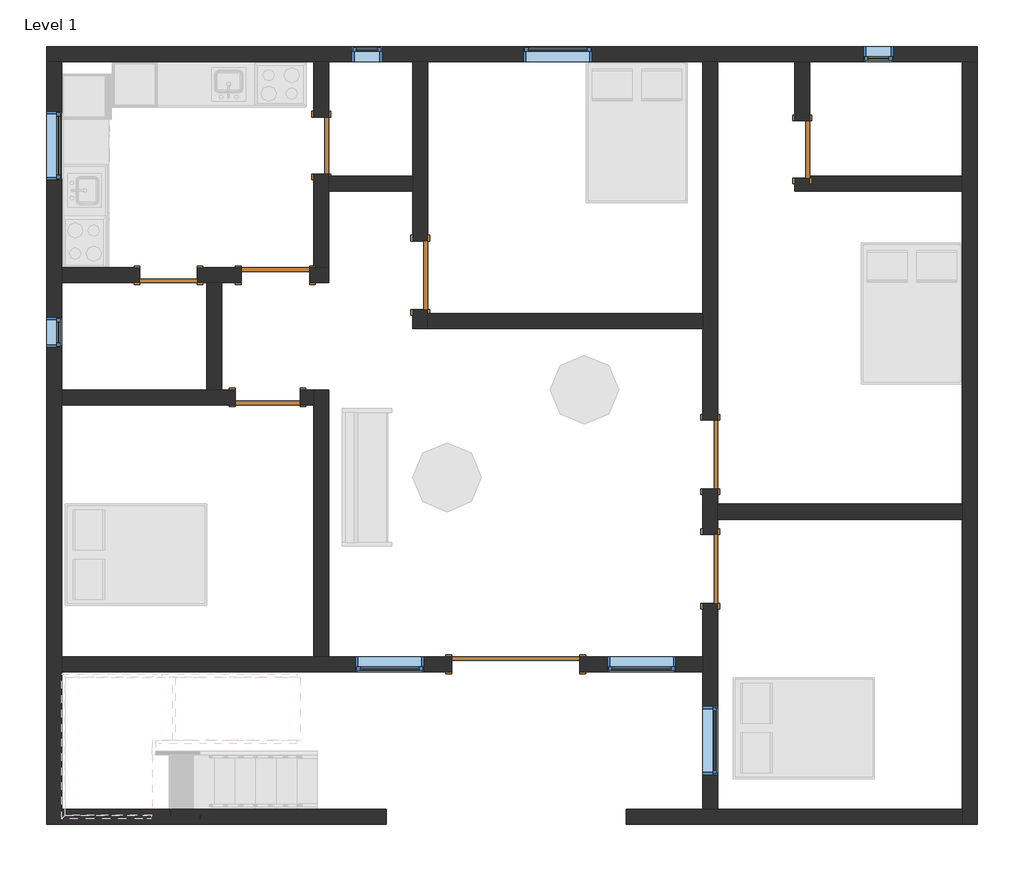
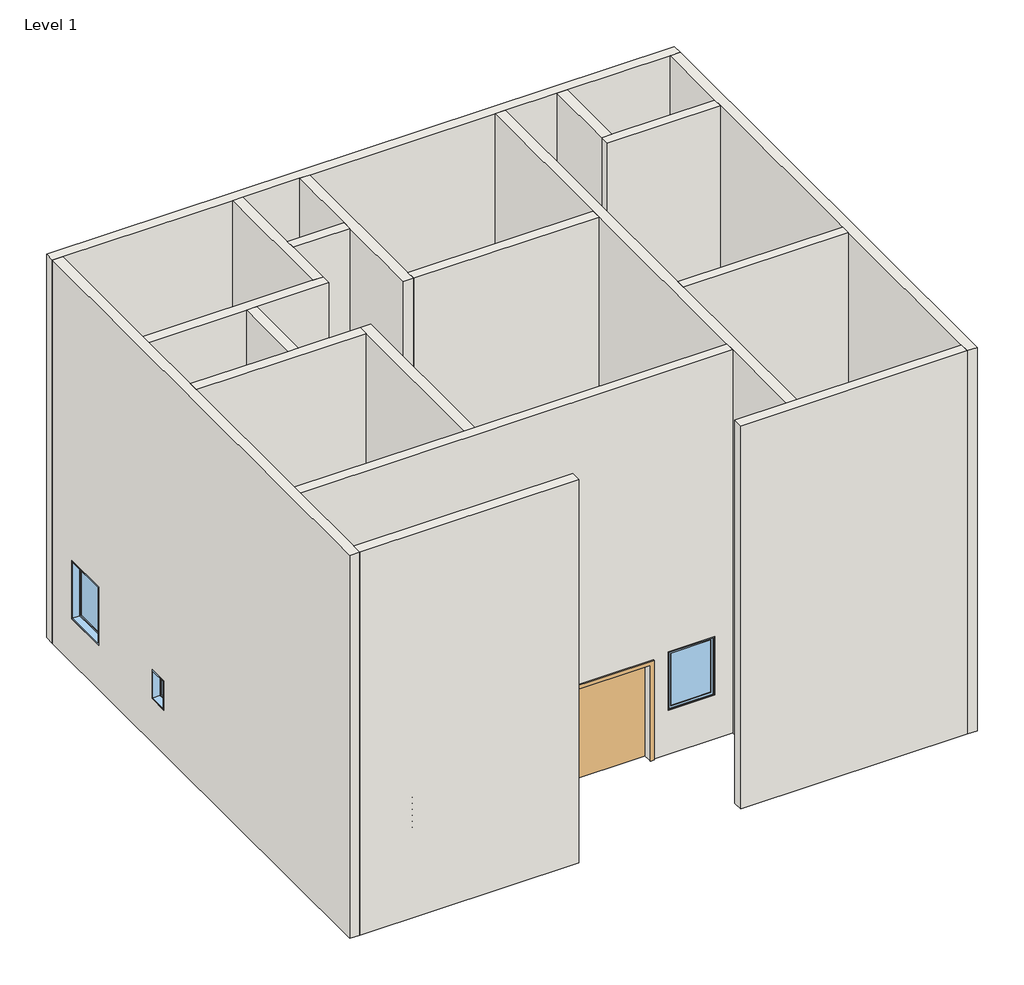
# One storey, part 1 of 4: 18 walls, 9 doors, 8 windows.
"""IFC4 building model written with IfcOpenShell, lengths in millimetres."""

from ifc_helpers import new_model, si_unit, frame, origin, origin_with_axes, place, context, project, spatial, polyline, outline, extrude, faceted_brep, transform, mapped, element, save
from components import m_door_double_flush_panel_double_acting_1700_x_2000mm_0a6d9c7f, m_single_flush_0762_x_2032mm_0c256fab, m_single_flush_0762_x_2032mm_7341a4fb, m_single_flush_0864_x_2032mm_0516f16c, m_single_flush_0915_x_2032mm_7267827e, m_single_flush_0915_x_2134mm_6a9e8738, m_single_flush_0915_x_2134mm_727434cd, m_fixed_0406_x_0610mm_8205b201, m_fixed_0915_x_0610mm_70a843a6, m_fixed_0915_x_1220mm_488fb2fb

model = new_model("IFC4")

# Units and contexts
model_context = context("Model", 3, world=origin())
ifc_project = project(units=[si_unit("LENGTHUNIT", "METRE", prefix="MILLI")], contexts=[model_context])

# Site, building, storey
site = spatial("IfcSite", under=ifc_project)
building = spatial("IfcBuilding", under=site)
storey = spatial("IfcBuildingStorey", under=building, Name="Level 1", Elevation=0.0)

# Doors
placement = place(None, origin())
m_door_double_flush_panel_double_acting_1700_x_2000mm_shape = m_door_double_flush_panel_double_acting_1700_x_2000mm_0a6d9c7f(model_context)
element("IfcDoor", 1, ObjectType="M_Door-Double-Flush_Panel-Double-Acting : 1700 x 2000mm", at=placement, inside=storey, context=model_context, shape_type="MappedRepresentation", body=[
    mapped(m_door_double_flush_panel_double_acting_1700_x_2000mm_shape, transform((-4513.6870075, 3420.4865734, 0.0), x_axis=(1.0, 0.0, 0.0), y_axis=(0.0, 1.0, 0.0), z_axis=(0.0, 0.0, 1.0))),
])
m_single_flush_0762_x_2032mm_shape = m_single_flush_0762_x_2032mm_0c256fab(model_context)
element("IfcDoor", 2, ObjectType="M_Single-Flush : 0762 x 2032mm", at=placement, inside=storey, context=model_context, shape_type="MappedRepresentation", body=[
    mapped(m_single_flush_0762_x_2032mm_shape, transform((-7102.8870075, 10329.2865734, 0.0), x_axis=(0.0, -1.0, 0.0), y_axis=(1.0, 0.0, 0.0), z_axis=(0.0, 0.0, 1.0))),
])
element("IfcDoor", 3, ObjectType="M_Single-Flush : 0762 x 2032mm", at=placement, inside=storey, context=model_context, shape_type="MappedRepresentation", body=[
    mapped(m_single_flush_0762_x_2032mm_shape, transform((-700.4870075, 10278.4865734, 0.0), x_axis=(0.0, -1.0, 0.0), y_axis=(1.0, 0.0, 0.0), z_axis=(0.0, 0.0, 1.0))),
])
m_single_flush_0762_x_2032mm_2_shape = m_single_flush_0762_x_2032mm_7341a4fb(model_context)
element("IfcDoor", 4, ObjectType="M_Single-Flush : 0762 x 2032mm", at=placement, inside=storey, context=model_context, shape_type="MappedRepresentation", body=[
    mapped(m_single_flush_0762_x_2032mm_2_shape, transform((-9136.4870075, 8602.0865734, 0.0), x_axis=(1.0, 0.0, 0.0), y_axis=(0.0, 1.0, 0.0), z_axis=(0.0, 0.0, 1.0))),
])
m_single_flush_0864_x_2032mm_shape = m_single_flush_0864_x_2032mm_0516f16c(model_context)
element("IfcDoor", 5, ObjectType="M_Single-Flush : 0864 x 2032mm", at=placement, inside=storey, context=model_context, shape_type="MappedRepresentation", body=[
    mapped(m_single_flush_0864_x_2032mm_shape, transform((-7815.6870075, 6976.4865734, 0.0), x_axis=(1.0, 0.0, 0.0), y_axis=(0.0, 1.0, 0.0), z_axis=(0.0, 0.0, 1.0))),
])
m_single_flush_0915_x_2032mm_shape = m_single_flush_0915_x_2032mm_7267827e(model_context)
element("IfcDoor", 6, ObjectType="M_Single-Flush : 0915 x 2032mm", at=placement, inside=storey, context=model_context, shape_type="MappedRepresentation", body=[
    mapped(m_single_flush_0915_x_2032mm_shape, transform((-5783.6870075, 8602.0865734, 0.0), x_axis=(0.0, -1.0, 0.0), y_axis=(1.0, 0.0, 0.0), z_axis=(0.0, 0.0, 1.0))),
])
m_single_flush_0915_x_2134mm_shape = m_single_flush_0915_x_2134mm_6a9e8738(model_context)
element("IfcDoor", 7, ObjectType="M_Single-Flush : 0915 x 2134mm", at=placement, inside=storey, context=model_context, shape_type="MappedRepresentation", body=[
    mapped(m_single_flush_0915_x_2134mm_shape, transform((-7712.4870075, 8602.0865734, 0.0), x_axis=(1.0, 0.0, 0.0), y_axis=(0.0, 1.0, 0.0), z_axis=(0.0, 0.0, 1.0))),
])
element("IfcDoor", 8, ObjectType="M_Single-Flush : 0915 x 2134mm", at=placement, inside=storey, context=model_context, shape_type="MappedRepresentation", body=[
    mapped(m_single_flush_0915_x_2134mm_shape, transform((-1922.8870075, 6214.4865734, 0.0), x_axis=(0.0, -1.0, 0.0), y_axis=(1.0, 0.0, 0.0), z_axis=(0.0, 0.0, 1.0))),
])
m_single_flush_0915_x_2134mm_2_shape = m_single_flush_0915_x_2134mm_727434cd(model_context)
element("IfcDoor", 9, ObjectType="M_Single-Flush : 0915 x 2134mm", at=placement, inside=storey, context=model_context, shape_type="MappedRepresentation", body=[
    mapped(m_single_flush_0915_x_2134mm_2_shape, transform((-1922.8870075, 4690.4865734, 0.0), x_axis=(0.0, 1.0, 0.0), y_axis=(-1.0, 0.0, 0.0), z_axis=(0.0, 0.0, 1.0))),
])

# Walls
element("IfcWall", 10, ObjectType="Generic - 200mm", at=placement, inside=storey, context=model_context, shape_type="Brep", body=[
    faceted_brep([(-10758.8870075, 11448.4865734, 0.0), (-10558.8870075, 11448.4865734, 0.0), (-7202.8870075, 11448.4865734, 0.0), (-7002.8870075, 11448.4865734, 0.0), (-5883.6870075, 11448.4865734, 0.0), (-5683.6870075, 11448.4865734, 0.0), (-2022.8870075, 11448.4865734, 0.0), (-1822.8870075, 11448.4865734, 0.0), (-800.4870075, 11448.4865734, 0.0), (-600.4870075, 11448.4865734, 0.0), (1433.1129925, 11448.4865734, 0.0), (1633.1129925, 11448.4865734, 0.0), (1633.1129925, 11448.4865734, 8000.0), (1433.1129925, 11448.4865734, 8000.0), (-600.4870075, 11448.4865734, 8000.0), (-800.4870075, 11448.4865734, 8000.0), (-1822.8870075, 11448.4865734, 8000.0), (-2022.8870075, 11448.4865734, 8000.0), (-5683.6870075, 11448.4865734, 8000.0), (-5883.6870075, 11448.4865734, 8000.0), (-7002.8870075, 11448.4865734, 8000.0), (-7202.8870075, 11448.4865734, 8000.0), (-10558.8870075, 11448.4865734, 8000.0), (-10758.8870075, 11448.4865734, 8000.0), (-4412.3870075, 11448.4865734, 915.0), (-4412.3870075, 11448.4865734, 1525.0), (-3497.3870075, 11448.4865734, 1525.0), (-3497.3870075, 11448.4865734, 915.0), (-6696.2870075, 11448.4865734, 915.0), (-6696.2870075, 11448.4865734, 1525.0), (-6290.2870075, 11448.4865734, 1525.0), (-6290.2870075, 11448.4865734, 915.0), (516.9129925, 11448.4865734, 915.0), (110.9129925, 11448.4865734, 915.0), (110.9129925, 11448.4865734, 1525.0), (516.9129925, 11448.4865734, 1525.0), (-10758.8870075, 11648.4865734, 0.0), (-10758.8870075, 11648.4865734, 8000.0), (1633.1129925, 11648.4865734, 8000.0), (1633.1129925, 11648.4865734, 0.0), (-4412.3870075, 11648.4865734, 915.0), (-3497.3870075, 11648.4865734, 915.0), (-3497.3870075, 11648.4865734, 1525.0), (-4412.3870075, 11648.4865734, 1525.0), (-6696.2870075, 11648.4865734, 915.0), (-6290.2870075, 11648.4865734, 915.0), (-6290.2870075, 11648.4865734, 1525.0), (-6696.2870075, 11648.4865734, 1525.0), (516.9129925, 11648.4865734, 915.0), (516.9129925, 11648.4865734, 1525.0), (110.9129925, 11648.4865734, 1525.0), (110.9129925, 11648.4865734, 915.0)], [[[0, 1, 2, 3, 4, 5, 6, 7, 8, 9, 10, 11, 12, 13, 14, 15, 16, 17, 18, 19, 20, 21, 22, 23], [24, 25, 26, 27], [28, 29, 30, 31], [32, 33, 34, 35]], [[36, 37, 38, 39], [40, 41, 42, 43], [44, 45, 46, 47], [48, 49, 50, 51]], [[11, 10, 9, 8, 7, 6, 5, 4, 3, 2, 1, 0, 36, 39]], [[23, 22, 21, 20, 19, 18, 17, 16, 15, 14, 13, 12, 38, 37]], [[12, 11, 39, 38]], [[0, 23, 37, 36]], [[25, 24, 40, 43]], [[26, 25, 43, 42]], [[27, 26, 42, 41]], [[24, 27, 41, 40]], [[29, 28, 44, 47]], [[30, 29, 47, 46]], [[31, 30, 46, 45]], [[28, 31, 45, 44]], [[49, 48, 32, 35]], [[50, 49, 35, 34]], [[51, 50, 34, 33]], [[48, 51, 33, 32]]]),
])
element("IfcWall", 11, ObjectType="Generic - 200mm", at=placement, inside=storey, context=model_context, shape_type="Brep", body=[
    faceted_brep([(1433.1129925, 11448.4865734, 0.0), (1433.1129925, 9921.2865734, 0.0), (1433.1129925, 9721.2865734, 0.0), (1433.1129925, 5552.4865734, 0.0), (1433.1129925, 5352.4865734, 0.0), (1433.1129925, 1488.4865734, 0.0), (1433.1129925, 1288.4865734, 0.0), (1433.1129925, 1288.4865734, 8000.0), (1433.1129925, 1488.4865734, 8000.0), (1433.1129925, 5352.4865734, 8000.0), (1433.1129925, 5552.4865734, 8000.0), (1433.1129925, 9721.2865734, 8000.0), (1433.1129925, 9921.2865734, 8000.0), (1433.1129925, 11448.4865734, 8000.0), (1633.1129925, 11448.4865734, 0.0), (1633.1129925, 11448.4865734, 8000.0), (1633.1129925, 1288.4865734, 8000.0), (1633.1129925, 1288.4865734, 0.0)], [[[0, 1, 2, 3, 4, 5, 6, 7, 8, 9, 10, 11, 12, 13]], [[14, 15, 16, 17]], [[6, 5, 4, 3, 2, 1, 0, 14, 17]], [[13, 12, 11, 10, 9, 8, 7, 16, 15]], [[0, 13, 15, 14]], [[7, 6, 17, 16]]]),
])
element("IfcWall", 12, ObjectType="Generic - 200mm", at=placement, inside=storey, context=model_context, shape_type="Brep", body=[
    faceted_brep([(-10558.8870075, 1288.4865734, 0.0), (-10558.8870075, 1488.4865734, 0.0), (-10558.8870075, 3320.4865734, 0.0), (-10558.8870075, 3520.4865734, 0.0), (-10558.8870075, 6876.4865734, 0.0), (-10558.8870075, 7076.4865734, 0.0), (-10558.8870075, 8502.0865734, 0.0), (-10558.8870075, 8702.0865734, 0.0), (-10558.8870075, 11448.4865734, 0.0), (-10558.8870075, 11448.4865734, 8000.0), (-10558.8870075, 8702.0865734, 8000.0), (-10558.8870075, 8502.0865734, 8000.0), (-10558.8870075, 7076.4865734, 8000.0), (-10558.8870075, 6876.4865734, 8000.0), (-10558.8870075, 3520.4865734, 8000.0), (-10558.8870075, 3320.4865734, 8000.0), (-10558.8870075, 1488.4865734, 8000.0), (-10558.8870075, 1288.4865734, 8000.0), (-10558.8870075, 10786.7865734, 915.0), (-10558.8870075, 9871.7865734, 915.0), (-10558.8870075, 9871.7865734, 2135.0), (-10558.8870075, 10786.7865734, 2135.0), (-10558.8870075, 8043.0865734, 915.0), (-10558.8870075, 7637.0865734, 915.0), (-10558.8870075, 7637.0865734, 1525.0), (-10558.8870075, 8043.0865734, 1525.0), (-10758.8870075, 1288.4865734, 0.0), (-10758.8870075, 1288.4865734, 8000.0), (-10758.8870075, 11448.4865734, 8000.0), (-10758.8870075, 11448.4865734, 0.0), (-10758.8870075, 10786.7865734, 915.0), (-10758.8870075, 10786.7865734, 2135.0), (-10758.8870075, 9871.7865734, 2135.0), (-10758.8870075, 9871.7865734, 915.0), (-10758.8870075, 8043.0865734, 915.0), (-10758.8870075, 8043.0865734, 1525.0), (-10758.8870075, 7637.0865734, 1525.0), (-10758.8870075, 7637.0865734, 915.0)], [[[0, 1, 2, 3, 4, 5, 6, 7, 8, 9, 10, 11, 12, 13, 14, 15, 16, 17], [18, 19, 20, 21], [22, 23, 24, 25]], [[26, 27, 28, 29], [30, 31, 32, 33], [34, 35, 36, 37]], [[8, 7, 6, 5, 4, 3, 2, 1, 0, 26, 29]], [[17, 16, 15, 14, 13, 12, 11, 10, 9, 28, 27]], [[9, 8, 29, 28]], [[31, 30, 18, 21]], [[32, 31, 21, 20]], [[33, 32, 20, 19]], [[30, 33, 19, 18]], [[35, 34, 22, 25]], [[36, 35, 25, 24]], [[37, 36, 24, 23]], [[34, 37, 23, 22]], [[0, 17, 27, 26]]]),
])
element("IfcWall", 13, ObjectType="Generic - 200mm", at=placement, inside=storey, context=model_context, shape_type="Brep", body=[
    faceted_brep([(-8755.4870075, 8502.0865734, 2032.0), (-8755.4870075, 8502.0865734, 0.0), (-8626.8870075, 8502.0865734, 0.0), (-8426.8870075, 8502.0865734, 0.0), (-8169.9870075, 8502.0865734, 0.0), (-8169.9870075, 8502.0865734, 2134.0), (-7254.9870075, 8502.0865734, 2134.0), (-7254.9870075, 8502.0865734, 0.0), (-7002.8870075, 8502.0865734, 0.0), (-7002.8870075, 8502.0865734, 8000.0), (-8426.8870075, 8502.0865734, 8000.0), (-8626.8870075, 8502.0865734, 8000.0), (-10558.8870075, 8502.0865734, 8000.0), (-10558.8870075, 8502.0865734, 0.0), (-9517.4870075, 8502.0865734, 0.0), (-9517.4870075, 8502.0865734, 2032.0), (-8169.9870075, 8702.0865734, 0.0), (-8755.4870075, 8702.0865734, 0.0), (-8755.4870075, 8702.0865734, 2032.0), (-9517.4870075, 8702.0865734, 2032.0), (-9517.4870075, 8702.0865734, 0.0), (-10558.8870075, 8702.0865734, 0.0), (-10558.8870075, 8702.0865734, 8000.0), (-7202.8870075, 8702.0865734, 8000.0), (-7002.8870075, 8702.0865734, 8000.0), (-7002.8870075, 8702.0865734, 0.0), (-7202.8870075, 8702.0865734, 0.0), (-7254.9870075, 8702.0865734, 0.0), (-7254.9870075, 8702.0865734, 2134.0), (-8169.9870075, 8702.0865734, 2134.0)], [[[0, 1, 2, 3, 4, 5, 6, 7, 8, 9, 10, 11, 12, 13, 14, 15]], [[16, 17, 18, 19, 20, 21, 22, 23, 24, 25, 26, 27, 28, 29]], [[8, 7, 27, 26, 25]], [[14, 13, 21, 20]], [[4, 3, 2, 1, 17, 16]], [[12, 11, 10, 9, 24, 23, 22]], [[13, 12, 22, 21]], [[9, 8, 25, 24]], [[28, 27, 7, 6]], [[29, 28, 6, 5]], [[16, 29, 5, 4]], [[18, 17, 1, 0]], [[19, 18, 0, 15]], [[20, 19, 15, 14]]]),
])
element("IfcWall", 14, ObjectType="Generic - 200mm", at=placement, inside=storey, context=model_context, shape_type="Brep", body=[
    faceted_brep([(-7002.8870075, 8702.0865734, 0.0), (-7002.8870075, 9721.2865734, 0.0), (-7002.8870075, 9921.2865734, 0.0), (-7002.8870075, 9948.2865734, 0.0), (-7002.8870075, 9948.2865734, 2032.0), (-7002.8870075, 10710.2865734, 2032.0), (-7002.8870075, 10710.2865734, 0.0), (-7002.8870075, 11448.4865734, 0.0), (-7002.8870075, 11448.4865734, 8000.0), (-7002.8870075, 9921.2865734, 8000.0), (-7002.8870075, 9721.2865734, 8000.0), (-7002.8870075, 8702.0865734, 8000.0), (-7202.8870075, 9948.2865734, 2032.0), (-7202.8870075, 9948.2865734, 0.0), (-7202.8870075, 8702.0865734, 0.0), (-7202.8870075, 8702.0865734, 8000.0), (-7202.8870075, 11448.4865734, 8000.0), (-7202.8870075, 11448.4865734, 0.0), (-7202.8870075, 10710.2865734, 0.0), (-7202.8870075, 10710.2865734, 2032.0)], [[[0, 1, 2, 3, 4, 5, 6, 7, 8, 9, 10, 11]], [[12, 13, 14, 15, 16, 17, 18, 19]], [[18, 17, 7, 6]], [[14, 13, 3, 2, 1, 0]], [[11, 10, 9, 8, 16, 15]], [[0, 11, 15, 14]], [[8, 7, 17, 16]], [[4, 3, 13, 12]], [[5, 4, 12, 19]], [[6, 5, 19, 18]]]),
])
element("IfcWall", 15, ObjectType="Generic - 200mm", at=placement, inside=storey, context=model_context, shape_type="SweptSolid", body=[
    extrude(outline(polyline([(-5883.6870075, 9721.2865734), (-7002.8870075, 9721.2865734), (-7002.8870075, 9921.2865734), (-5883.6870075, 9921.2865734), (-5883.6870075, 9721.2865734)])), origin_with_axes(), (0.0, 0.0, 1.0), 8000.0),
])
element("IfcWall", 16, ObjectType="Generic - 200mm", at=placement, inside=storey, context=model_context, shape_type="Brep", body=[
    faceted_brep([(-5683.6870075, 7892.4865734, 0.0), (-5683.6870075, 8092.4865734, 0.0), (-5683.6870075, 8144.5865734, 0.0), (-5683.6870075, 8144.5865734, 2032.0), (-5683.6870075, 9059.5865734, 2032.0), (-5683.6870075, 9059.5865734, 0.0), (-5683.6870075, 11448.4865734, 0.0), (-5683.6870075, 11448.4865734, 8000.0), (-5683.6870075, 8092.4865734, 8000.0), (-5683.6870075, 7892.4865734, 8000.0), (-5883.6870075, 8144.5865734, 2032.0), (-5883.6870075, 8144.5865734, 0.0), (-5883.6870075, 7892.4865734, 0.0), (-5883.6870075, 7892.4865734, 8000.0), (-5883.6870075, 9721.2865734, 8000.0), (-5883.6870075, 9921.2865734, 8000.0), (-5883.6870075, 11448.4865734, 8000.0), (-5883.6870075, 11448.4865734, 0.0), (-5883.6870075, 9921.2865734, 0.0), (-5883.6870075, 9721.2865734, 0.0), (-5883.6870075, 9059.5865734, 0.0), (-5883.6870075, 9059.5865734, 2032.0)], [[[0, 1, 2, 3, 4, 5, 6, 7, 8, 9]], [[10, 11, 12, 13, 14, 15, 16, 17, 18, 19, 20, 21]], [[12, 11, 2, 1, 0]], [[20, 19, 18, 17, 6, 5]], [[9, 8, 7, 16, 15, 14, 13]], [[7, 6, 17, 16]], [[0, 9, 13, 12]], [[3, 2, 11, 10]], [[4, 3, 10, 21]], [[5, 4, 21, 20]]]),
])
element("IfcWall", 17, ObjectType="Generic - 200mm", at=placement, inside=storey, context=model_context, shape_type="SweptSolid", body=[
    extrude(outline(polyline([(-2022.8870075, 7892.4865734), (-5683.6870075, 7892.4865734), (-5683.6870075, 8092.4865734), (-2022.8870075, 8092.4865734), (-2022.8870075, 7892.4865734)])), origin_with_axes(), (0.0, 0.0, 1.0), 8000.0),
])
element("IfcWall", 18, ObjectType="Generic - 200mm", at=placement, inside=storey, context=model_context, shape_type="Brep", body=[
    faceted_brep([(-800.4870075, 9921.2865734, 8000.0), (-600.4870075, 9921.2865734, 8000.0), (1433.1129925, 9921.2865734, 8000.0), (1433.1129925, 9921.2865734, 0.0), (-600.4870075, 9921.2865734, 0.0), (-600.4870075, 9921.2865734, 2032.0), (-800.4870075, 9921.2865734, 2032.0), (-800.4870075, 9721.2865734, 0.0), (1433.1129925, 9721.2865734, 0.0), (1433.1129925, 9721.2865734, 8000.0), (-800.4870075, 9721.2865734, 8000.0), (-800.4870075, 9897.4865734, 0.0), (-600.4870075, 9897.4865734, 0.0), (-800.4870075, 9897.4865734, 2032.0), (-600.4870075, 9897.4865734, 2032.0)], [[[0, 1, 2, 3, 4, 5, 6]], [[7, 8, 9, 10]], [[8, 7, 11, 12, 4, 3]], [[2, 1, 0, 10, 9]], [[3, 2, 9, 8]], [[7, 10, 0, 6, 13, 11]], [[12, 14, 5, 4]], [[14, 12, 11, 13]], [[14, 13, 6, 5]]]),
])
element("IfcWall", 19, ObjectType="Generic - 200mm", at=placement, inside=storey, context=model_context, shape_type="SweptSolid", body=[
    extrude(outline(polyline([(9921.2865734, 8000.0), (11448.4865734, 8000.0), (11448.4865734, 0.0), (10659.4865734, 0.0), (10659.4865734, 2032.0), (9921.2865734, 2032.0), (9921.2865734, 8000.0)])), frame((-800.4870075, 0.0, 0.0), z_axis=(1.0, 0.0, 0.0), x_axis=(0.0, 1.0, 0.0)), (0.0, 0.0, 1.0), 200.0),
])
element("IfcWall", 20, ObjectType="Generic - 200mm", at=placement, inside=storey, context=model_context, shape_type="Brep", body=[
    faceted_brep([(-1822.8870075, 5147.9865734, 2134.0), (-1822.8870075, 5147.9865734, 0.0), (-1822.8870075, 5352.4865734, 0.0), (-1822.8870075, 5552.4865734, 0.0), (-1822.8870075, 5756.9865734, 0.0), (-1822.8870075, 5756.9865734, 2134.0), (-1822.8870075, 6671.9865734, 2134.0), (-1822.8870075, 6671.9865734, 0.0), (-1822.8870075, 11448.4865734, 0.0), (-1822.8870075, 11448.4865734, 8000.0), (-1822.8870075, 5552.4865734, 8000.0), (-1822.8870075, 5352.4865734, 8000.0), (-1822.8870075, 1488.4865734, 8000.0), (-1822.8870075, 1488.4865734, 0.0), (-1822.8870075, 4232.9865734, 0.0), (-1822.8870075, 4232.9865734, 2134.0), (-1822.8870075, 2861.9865734, 915.0), (-1822.8870075, 1946.9865734, 915.0), (-1822.8870075, 1946.9865734, 2135.0), (-1822.8870075, 2861.9865734, 2135.0), (-2022.8870075, 5756.9865734, 0.0), (-2022.8870075, 5147.9865734, 0.0), (-2022.8870075, 5147.9865734, 2134.0), (-2022.8870075, 4232.9865734, 2134.0), (-2022.8870075, 4232.9865734, 0.0), (-2022.8870075, 3520.4865734, 0.0), (-2022.8870075, 3320.4865734, 0.0), (-2022.8870075, 1488.4865734, 0.0), (-2022.8870075, 1488.4865734, 8000.0), (-2022.8870075, 3320.4865734, 8000.0), (-2022.8870075, 3520.4865734, 8000.0), (-2022.8870075, 7892.4865734, 8000.0), (-2022.8870075, 8092.4865734, 8000.0), (-2022.8870075, 11448.4865734, 8000.0), (-2022.8870075, 11448.4865734, 0.0), (-2022.8870075, 8092.4865734, 0.0), (-2022.8870075, 7892.4865734, 0.0), (-2022.8870075, 6671.9865734, 0.0), (-2022.8870075, 6671.9865734, 2134.0), (-2022.8870075, 5756.9865734, 2134.0), (-2022.8870075, 2861.9865734, 915.0), (-2022.8870075, 2861.9865734, 2135.0), (-2022.8870075, 1946.9865734, 2135.0), (-2022.8870075, 1946.9865734, 915.0)], [[[0, 1, 2, 3, 4, 5, 6, 7, 8, 9, 10, 11, 12, 13, 14, 15], [16, 17, 18, 19]], [[20, 21, 22, 23, 24, 25, 26, 27, 28, 29, 30, 31, 32, 33, 34, 35, 36, 37, 38, 39], [40, 41, 42, 43]], [[37, 36, 35, 34, 8, 7]], [[14, 13, 27, 26, 25, 24]], [[4, 3, 2, 1, 21, 20]], [[12, 11, 10, 9, 33, 32, 31, 30, 29, 28]], [[9, 8, 34, 33]], [[5, 4, 20, 39]], [[6, 5, 39, 38]], [[7, 6, 38, 37]], [[22, 21, 1, 0]], [[23, 22, 0, 15]], [[24, 23, 15, 14]], [[41, 40, 16, 19]], [[42, 41, 19, 18]], [[43, 42, 18, 17]], [[40, 43, 17, 16]], [[13, 12, 28, 27]]]),
])
element("IfcWall", 21, ObjectType="Generic - 200mm", at=placement, inside=storey, context=model_context, shape_type="SweptSolid", body=[
    extrude(outline(polyline([(1433.1129925, 5352.4865734), (-1822.8870075, 5352.4865734), (-1822.8870075, 5552.4865734), (1433.1129925, 5552.4865734), (1433.1129925, 5352.4865734)])), origin_with_axes(), (0.0, 0.0, 1.0), 8000.0),
])
element("IfcWall", 22, ObjectType="Generic - 200mm", at=placement, inside=storey, context=model_context, shape_type="Brep", body=[
    faceted_brep([(-7383.6870075, 6876.4865734, 2032.0), (-7383.6870075, 6876.4865734, 0.0), (-7204.4870075, 6876.4865734, 0.0), (-7204.4870075, 6876.4865734, 8000.0), (-10558.8870075, 6876.4865734, 8000.0), (-10558.8870075, 6876.4865734, 0.0), (-8247.6870075, 6876.4865734, 0.0), (-8247.6870075, 6876.4865734, 2032.0), (-7204.4870075, 7076.4865734, 0.0), (-7383.6870075, 7076.4865734, 0.0), (-7383.6870075, 7076.4865734, 2032.0), (-8247.6870075, 7076.4865734, 2032.0), (-8247.6870075, 7076.4865734, 0.0), (-8426.8870075, 7076.4865734, 0.0), (-8626.8870075, 7076.4865734, 0.0), (-10558.8870075, 7076.4865734, 0.0), (-10558.8870075, 7076.4865734, 8000.0), (-8626.8870075, 7076.4865734, 8000.0), (-8426.8870075, 7076.4865734, 8000.0), (-7204.4870075, 7076.4865734, 8000.0)], [[[0, 1, 2, 3, 4, 5, 6, 7]], [[8, 9, 10, 11, 12, 13, 14, 15, 16, 17, 18, 19]], [[6, 5, 15, 14, 13, 12]], [[2, 1, 9, 8]], [[4, 3, 19, 18, 17, 16]], [[5, 4, 16, 15]], [[3, 2, 8, 19]], [[10, 9, 1, 0]], [[11, 10, 0, 7]], [[12, 11, 7, 6]]]),
])
element("IfcWall", 23, ObjectType="Generic - 200mm", at=placement, inside=storey, context=model_context, shape_type="SweptSolid", body=[
    extrude(outline(polyline([(-8426.8870075, 8502.0865734), (-8426.8870075, 7076.4865734), (-8626.8870075, 7076.4865734), (-8626.8870075, 8502.0865734), (-8426.8870075, 8502.0865734)])), origin_with_axes(), (0.0, 0.0, 1.0), 8000.0),
])
element("IfcWall", 24, ObjectType="Generic - 200mm", at=placement, inside=storey, context=model_context, shape_type="Brep", body=[
    faceted_brep([(-2022.8870075, 3320.4865734, 8000.0), (-10558.8870075, 3320.4865734, 8000.0), (-10558.8870075, 3320.4865734, 0.0), (-5363.6870075, 3320.4865734, 0.0), (-5363.6870075, 3320.4865734, 2000.0), (-3663.6870075, 3320.4865734, 2000.0), (-3663.6870075, 3320.4865734, 0.0), (-2022.8870075, 3320.4865734, 0.0), (-5732.5870075, 3320.4865734, 915.0), (-6647.5870075, 3320.4865734, 915.0), (-6647.5870075, 3320.4865734, 2135.0), (-5732.5870075, 3320.4865734, 2135.0), (-2379.7870075, 3320.4865734, 915.0), (-3294.7870075, 3320.4865734, 915.0), (-3294.7870075, 3320.4865734, 2135.0), (-2379.7870075, 3320.4865734, 2135.0), (-10558.8870075, 3520.4865734, 8000.0), (-7204.4870075, 3520.4865734, 8000.0), (-7004.4870075, 3520.4865734, 8000.0), (-2022.8870075, 3520.4865734, 8000.0), (-2022.8870075, 3520.4865734, 0.0), (-3663.6870075, 3520.4865734, 0.0), (-3663.6870075, 3520.4865734, 2000.0), (-5363.6870075, 3520.4865734, 2000.0), (-5363.6870075, 3520.4865734, 0.0), (-7004.4870075, 3520.4865734, 0.0), (-7204.4870075, 3520.4865734, 0.0), (-10558.8870075, 3520.4865734, 0.0), (-5732.5870075, 3520.4865734, 915.0), (-5732.5870075, 3520.4865734, 2135.0), (-6647.5870075, 3520.4865734, 2135.0), (-6647.5870075, 3520.4865734, 915.0), (-2379.7870075, 3520.4865734, 915.0), (-2379.7870075, 3520.4865734, 2135.0), (-3294.7870075, 3520.4865734, 2135.0), (-3294.7870075, 3520.4865734, 915.0)], [[[0, 1, 2, 3, 4, 5, 6, 7], [8, 9, 10, 11], [12, 13, 14, 15]], [[16, 17, 18, 19, 20, 21, 22, 23, 24, 25, 26, 27], [28, 29, 30, 31], [32, 33, 34, 35]], [[2, 27, 26, 25, 24, 3]], [[20, 7, 6, 21]], [[1, 0, 19, 18, 17, 16]], [[2, 1, 16, 27]], [[0, 7, 20, 19]], [[5, 22, 21, 6]], [[22, 5, 4, 23]], [[23, 4, 3, 24]], [[29, 28, 8, 11]], [[30, 29, 11, 10]], [[31, 30, 10, 9]], [[28, 31, 9, 8]], [[33, 32, 12, 15]], [[34, 33, 15, 14]], [[35, 34, 14, 13]], [[32, 35, 13, 12]]]),
])
element("IfcWall", 25, ObjectType="Generic - 200mm", at=placement, inside=storey, context=model_context, shape_type="Brep", body=[
    faceted_brep([(-7004.4870075, 3520.4865734, 0.0), (-7004.4870075, 7076.4865734, 0.0), (-7004.4870075, 7076.4865734, 8000.0), (-7004.4870075, 3520.4865734, 8000.0), (-7204.4870075, 3520.4865734, 0.0), (-7204.4870075, 3520.4865734, 8000.0), (-7204.4870075, 6876.4865734, 8000.0), (-7204.4870075, 7076.4865734, 8000.0), (-7204.4870075, 7076.4865734, 0.0), (-7204.4870075, 6876.4865734, 0.0)], [[[0, 1, 2, 3]], [[4, 5, 6, 7, 8, 9]], [[1, 0, 4, 9, 8]], [[3, 2, 7, 6, 5]], [[0, 3, 5, 4]], [[2, 1, 8, 7]]]),
])
element("IfcWall", 26, ObjectType="Generic - 200mm", at=placement, inside=storey, context=model_context, shape_type="SweptSolid", body=[
    extrude(outline(polyline([(-6239.2870075, 1288.4865734), (-10558.8870075, 1288.4865734), (-10558.8870075, 1488.4865734), (-6239.2870075, 1488.4865734), (-6239.2870075, 1288.4865734)])), origin_with_axes(), (0.0, 0.0, 1.0), 8000.0),
])
element("IfcWall", 27, ObjectType="Generic - 200mm", at=placement, inside=storey, context=model_context, shape_type="Brep", body=[
    faceted_brep([(1433.1129925, 1488.4865734, 0.0), (-1822.8870075, 1488.4865734, 0.0), (-2022.8870075, 1488.4865734, 0.0), (-3038.8870075, 1488.4865734, 0.0), (-3038.8870075, 1488.4865734, 8000.0), (-2022.8870075, 1488.4865734, 8000.0), (-1822.8870075, 1488.4865734, 8000.0), (1433.1129925, 1488.4865734, 8000.0), (1433.1129925, 1288.4865734, 0.0), (1433.1129925, 1288.4865734, 8000.0), (-3038.8870075, 1288.4865734, 8000.0), (-3038.8870075, 1288.4865734, 0.0)], [[[0, 1, 2, 3, 4, 5, 6, 7]], [[8, 9, 10, 11]], [[3, 2, 1, 0, 8, 11]], [[4, 3, 11, 10]], [[7, 6, 5, 4, 10, 9]], [[0, 7, 9, 8]]]),
])

# Windows
m_fixed_0406_x_0610mm_shape = m_fixed_0406_x_0610mm_8205b201(model_context)
element("IfcWindow", 28, ObjectType="M_Fixed : 0406 x 0610mm", at=placement, inside=storey, context=model_context, shape_type="MappedRepresentation", body=[
    mapped(m_fixed_0406_x_0610mm_shape, transform((-6493.2870075, 11535.4865734, 0.0), x_axis=(1.0, 0.0, 0.0), y_axis=(0.0, 1.0, 0.0), z_axis=(0.0, 0.0, 1.0))),
])
element("IfcWindow", 29, ObjectType="M_Fixed : 0406 x 0610mm", at=placement, inside=storey, context=model_context, shape_type="MappedRepresentation", body=[
    mapped(m_fixed_0406_x_0610mm_shape, transform((-10671.8870075, 7840.0865734, 0.0), x_axis=(0.0, -1.0, 0.0), y_axis=(1.0, 0.0, 0.0), z_axis=(0.0, 0.0, 1.0))),
])
element("IfcWindow", 30, ObjectType="M_Fixed : 0406 x 0610mm", at=placement, inside=storey, context=model_context, shape_type="MappedRepresentation", body=[
    mapped(m_fixed_0406_x_0610mm_shape, transform((313.9129925, 11561.4865734, 0.0), x_axis=(-1.0, 0.0, 0.0), y_axis=(0.0, -1.0, 0.0), z_axis=(0.0, 0.0, 1.0))),
])
m_fixed_0915_x_0610mm_shape = m_fixed_0915_x_0610mm_70a843a6(model_context)
element("IfcWindow", 31, ObjectType="M_Fixed : 0915 x 0610mm", at=placement, inside=storey, context=model_context, shape_type="MappedRepresentation", body=[
    mapped(m_fixed_0915_x_0610mm_shape, transform((-3954.8870075, 11535.4865734, 0.0), x_axis=(1.0, 0.0, 0.0), y_axis=(0.0, 1.0, 0.0), z_axis=(0.0, 0.0, 1.0))),
])
m_fixed_0915_x_1220mm_shape = m_fixed_0915_x_1220mm_488fb2fb(model_context)
element("IfcWindow", 32, ObjectType="M_Fixed : 0915 x 1220mm", at=placement, inside=storey, context=model_context, shape_type="MappedRepresentation", body=[
    mapped(m_fixed_0915_x_1220mm_shape, transform((-10671.8870075, 10329.2865734, 0.0), x_axis=(0.0, -1.0, 0.0), y_axis=(1.0, 0.0, 0.0), z_axis=(0.0, 0.0, 1.0))),
])
element("IfcWindow", 33, ObjectType="M_Fixed : 0915 x 1220mm", at=placement, inside=storey, context=model_context, shape_type="MappedRepresentation", body=[
    mapped(m_fixed_0915_x_1220mm_shape, transform((-6190.0870075, 3433.4865734, 0.0), x_axis=(-1.0, 0.0, 0.0), y_axis=(0.0, -1.0, 0.0), z_axis=(0.0, 0.0, 1.0))),
])
element("IfcWindow", 34, ObjectType="M_Fixed : 0915 x 1220mm", at=placement, inside=storey, context=model_context, shape_type="MappedRepresentation", body=[
    mapped(m_fixed_0915_x_1220mm_shape, transform((-2837.2870075, 3433.4865734, 0.0), x_axis=(-1.0, 0.0, 0.0), y_axis=(0.0, -1.0, 0.0), z_axis=(0.0, 0.0, 1.0))),
])
element("IfcWindow", 35, ObjectType="M_Fixed : 0915 x 1220mm", at=placement, inside=storey, context=model_context, shape_type="MappedRepresentation", body=[
    mapped(m_fixed_0915_x_1220mm_shape, transform((-1935.8870075, 2404.4865734, 0.0), x_axis=(0.0, -1.0, 0.0), y_axis=(1.0, 0.0, 0.0), z_axis=(0.0, 0.0, 1.0))),
])

save(model, "model.ifc")

# Revit data of these elements
# Type "M_Door-Double-Flush_Panel-Double-Acting : 1700 x 2000mm"
#   Type Mark = "22"
#   Construction Type Id = "DOOR"
#   Assembly Code = "C1020"
#   Analytic Construction = "Wooden"
#   W = 850 mm
#   Thickness = 50 mm
#   Thermal Resistance (R) = 0.455703 (m²·K)/W
#   Swing Angle [instance default] = 90.00°
#   Heat Transfer Coefficient (U) = 2.19465 W/(m²·K)
#   Height = 2000 mm
#   Trim Projection Ext. = 25 mm
#   Trim Projection Int. = 25 mm
#   Trim Width Ext. = 80 mm
#   Trim Width Int. = 80 mm
#   Width = 1700 mm
#   Define Thermal Properties by = 1
#   Panel Material = Wood - Birch - Solid Stained Light Low Gloss
#   Trim Material = Paint - Sienna
#   Visual Light Transmittance = 0
#   Solar Heat Gain Coefficient = 0
#   Function = (empty or 0)
#   Wall Closure = (empty or 0)
# Type "M_Single-Flush : 0762 x 2032mm"
#   Type Mark = "19"
#   Thickness = 51 mm
#   Height = 2032 mm
#   Trim Projection Ext = 25 mm
#   Trim Projection Int = 25 mm
#   Trim Width = 76 mm
#   Width = 762 mm
#   Door Material = Door - Panel
#   Frame Material = Door - Frame
#   Function = (empty or 0)
#   Wall Closure = (empty or 0)
# Type "M_Single-Flush : 0864 x 2032mm"
#   Type Mark = "21"
#   Thickness = 51 mm
#   Height = 2032 mm
#   Trim Projection Ext = 25 mm
#   Trim Projection Int = 25 mm
#   Trim Width = 76 mm
#   Width = 864 mm
#   Door Material = Door - Panel
#   Frame Material = Door - Frame
#   Function = (empty or 0)
#   Wall Closure = (empty or 0)
# Type "M_Single-Flush : 0915 x 2032mm"
#   Type Mark = "20"
#   Thickness = 51 mm
#   Height = 2032 mm
#   Trim Projection Ext = 25 mm
#   Trim Projection Int = 25 mm
#   Trim Width = 76 mm
#   Width = 915 mm
#   Door Material = Door - Panel
#   Frame Material = Door - Frame
#   Function = (empty or 0)
#   Wall Closure = (empty or 0)
# Type "M_Single-Flush : 0915 x 2134mm"
#   Type Mark = "15"
#   Thickness = 51 mm
#   Height = 2134 mm
#   Trim Projection Ext = 25 mm
#   Trim Projection Int = 25 mm
#   Trim Width = 76 mm
#   Width = 915 mm
#   Door Material = Door - Panel
#   Frame Material = Door - Frame
#   Function = (empty or 0)
#   Wall Closure = (empty or 0)
# Type "Generic - 200mm"
#   Layers, outside or top first: 200 mm no material (function 1)
# Type "M_Fixed : 0406 x 0610mm"
#   Type Mark = "10"
#   Height = 610 mm
#   Default Sill Height = 915 mm
#   Width = 406 mm
#   Window Inset = 19 mm
#   Frame Exterior Material = Sash
#   Frame Interior Material = Sash
#   Glass Pane Material = Glass
#   Sash = Sash
#   Wall Closure = (empty or 0)
# Type "M_Fixed : 0915 x 0610mm"
#   Type Mark = "14"
#   Height = 610 mm
#   Default Sill Height = 915 mm
#   Width = 915 mm
#   Window Inset = 19 mm
#   Frame Exterior Material = Sash
#   Frame Interior Material = Sash
#   Glass Pane Material = Glass
#   Sash = Sash
#   Wall Closure = (empty or 0)
# Type "M_Fixed : 0915 x 1220mm"
#   Type Mark = "15"
#   Height = 1220 mm
#   Default Sill Height = 915 mm
#   Width = 915 mm
#   Window Inset = 19 mm
#   Frame Exterior Material = Sash
#   Frame Interior Material = Sash
#   Glass Pane Material = Glass
#   Sash = Sash
#   Wall Closure = (empty or 0)
# Element 1 (IfcDoor, "M_Door-Double-Flush_Panel-Double-Acting : 1700 x 2000mm")
#   Swing Angle = 90.00°
#   Phase Created = New Construction
#   Materials on its faces: "Paint - Sienna", "Wood - Birch - Solid Stained Light Low Gloss"
# Elements 2, 3, 4 (IfcDoor, "M_Single-Flush : 0762 x 2032mm")
#   Phase Created = New Construction
#   Materials on its faces: "Door - Frame", "Door - Panel"
# Element 5 (IfcDoor, "M_Single-Flush : 0864 x 2032mm")
#   Phase Created = New Construction
#   Materials on its faces: "Door - Frame", "Door - Panel"
# Element 6 (IfcDoor, "M_Single-Flush : 0915 x 2032mm")
#   Phase Created = New Construction
#   Materials on its faces: "Door - Frame", "Door - Panel"
# Elements 7, 8, 9 (IfcDoor, "M_Single-Flush : 0915 x 2134mm")
#   Phase Created = New Construction
#   Materials on its faces: "Door - Frame", "Door - Panel"
# Elements 10, 11, 12, 13, 14, 15, 16, 17, 18, 19, 20, 21, 22, 23, 24, 25, 26, 27 (IfcWall, "Generic - 200mm")
#   Top Offset = 0 mm
#   Base Offset = 0 mm
#   Unconnected Height = 8000 mm
#   wall height = 8000 mm
#   Phase Created = New Construction
#   Base Constraint = Level 1
#   Materials on its faces: "Default Wall"
# Element 28 (IfcWindow, "M_Fixed : 0406 x 0610mm")
#   Mark = "7"
#   Phase Created = New Construction
#   Materials on its faces: "Sash", "Glass"
# Element 29 (IfcWindow, "M_Fixed : 0406 x 0610mm")
#   Mark = "9"
#   Phase Created = New Construction
#   Materials on its faces: "Sash", "Glass"
# Element 30 (IfcWindow, "M_Fixed : 0406 x 0610mm")
#   Mark = "10"
#   Phase Created = New Construction
#   Materials on its faces: "Sash", "Glass"
# Element 31 (IfcWindow, "M_Fixed : 0915 x 0610mm")
#   Mark = "6"
#   Phase Created = New Construction
#   Materials on its faces: "Sash", "Glass"
# Element 32 (IfcWindow, "M_Fixed : 0915 x 1220mm")
#   Mark = "8"
#   Phase Created = New Construction
#   Materials on its faces: "Sash", "Glass"
# Element 33 (IfcWindow, "M_Fixed : 0915 x 1220mm")
#   Mark = "11"
#   Phase Created = New Construction
#   Materials on its faces: "Sash", "Glass"
# Element 34 (IfcWindow, "M_Fixed : 0915 x 1220mm")
#   Mark = "12"
#   Phase Created = New Construction
#   Materials on its faces: "Sash", "Glass"
# Element 35 (IfcWindow, "M_Fixed : 0915 x 1220mm")
#   Mark = "13"
#   Phase Created = New Construction
#   Materials on its faces: "Sash", "Glass"
# Materials
#   "Wood - Birch - Solid Stained Light Low Gloss": class "Wood", colour RGB 210 159 95, transparency 0, Cost = 0
#   "Paint - Sienna": colour RGB 118 70 51, transparency 0, Cost = 0
#   "Door - Panel": class "Wood", colour RGB 114 82 51, transparency 0
#   "Door - Frame": colour RGB 153 76 43, transparency 0
#   "Sash": class "Wood", colour RGB 136 99 55, transparency 0
#   "Glass": class "Glass", colour RGB 218 227 224, transparency 0.85, Description = "Soda Lime Glass", Cost = 0
#   "Default Wall": colour RGB 80 80 80, transparency 0
